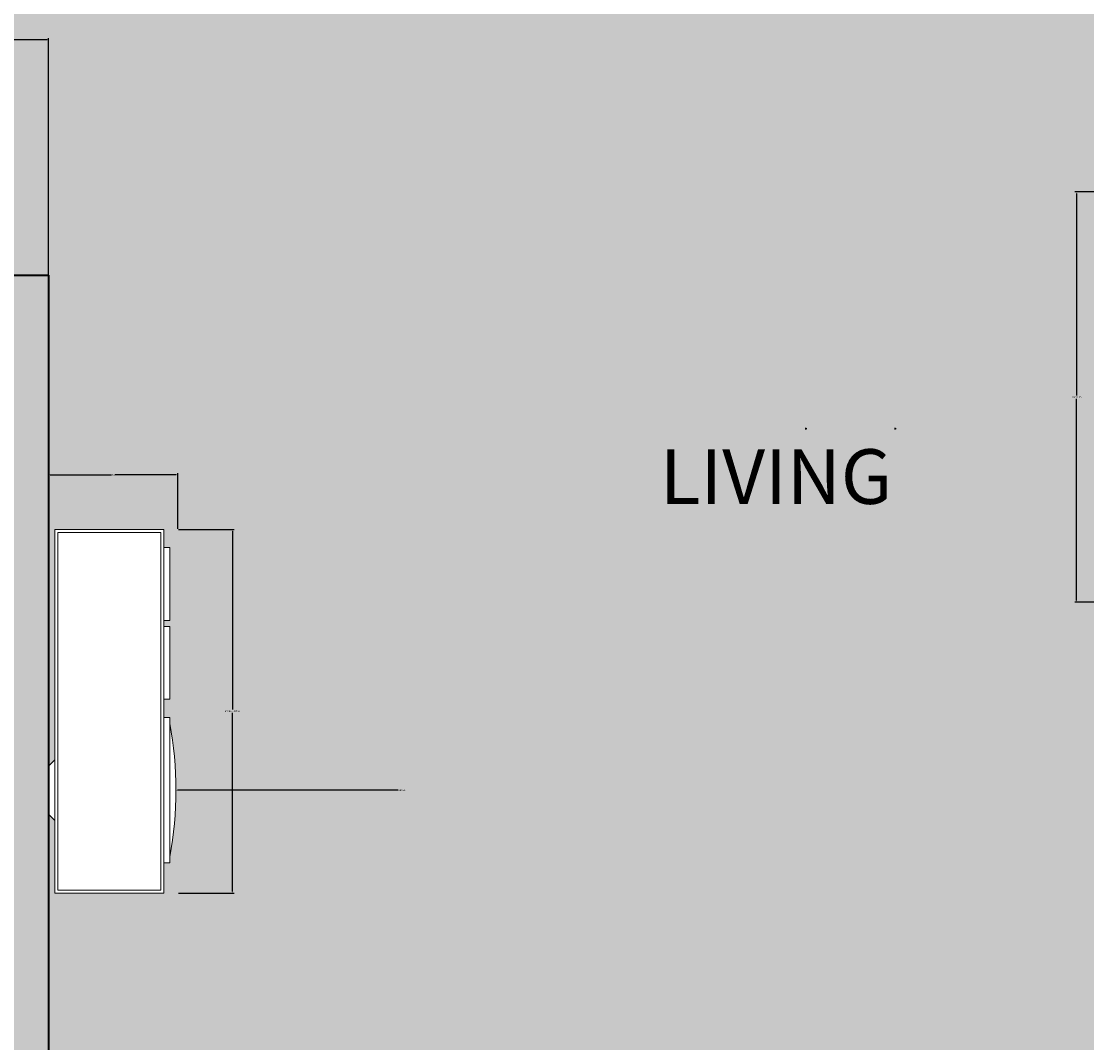
# Model space of a CAD drawing. Units: inches. Extents: x 3024 to 3952, y 1308 to 1863.
# Tile 5 of 29: x 3275 to 3392, y 1449 to 1560. Entities that reach past the tile are written whole.
import ezdxf

# ---------------------------------------------------------------- set-up
doc = ezdxf.new("R2010")
doc.units = ezdxf.units.IN
for name, color, linetype, lineweight in [('A-ANNO-DIMS', 2, 'Continuous', 18), ('A-AREA-IDEN', 7, 'Continuous', 18), ('A-FLOR-TILE-PATT', 7, 'Continuous', 13), ('A-FURN', 8, 'Continuous', 18), ('A-WALL', 7, 'Continuous', 35)]:
    doc.layers.add(name, color=color, linetype=linetype, lineweight=lineweight)
doc.layers.add('A-FLOR-PATT', color=254, linetype='Continuous', lineweight=13, true_color=0xfeeab9)
doc.layers.add('A-WALL-PATT', color=254, linetype='Continuous', lineweight=13, true_color=0xcecce6)
doc.styles.get("Standard").update_dxf_attribs({"font": 'arial.ttf'})
doc.dimstyles.get("Standard").update_dxf_attribs({"dimtxt": 0.18, "dimasz": 0.18, "dimexe": 0.18, "dimexo": 0.0625, "dimgap": 0.09, "dimtad": 0, "dimtih": 1, "dimtoh": 1, "dimdec": 4, "dimzin": 0, "dimdsep": 46, "dimtxsty": 'Standard', "dimcen": 0.09, "dimadec": 0, "dimazin": 0, "dimtfac": 1, "dimtdec": 4, "dimtofl": 0, "dimtmove": 0, "dimatfit": 3, "dimfxl": 1, "dimtolj": 1, "dimtzin": 0, "dimarcsym": 0})

# ---------------------------------------------------------------- blocks, each defined once
blk = doc.blocks.new('Entertainment Center')
for p, q in [((-4, 0), (-5, -1)), ((4, 0), (-4, 0)), ((5, -1), (4, 0)), ((-17, -19), (-17, -1)), ((-17, -1), (43, -1)), ((-16.5, -18.5), (-16.5, -1.5)), ((-16.5, -1.5), (42.5, -1.5)), ((42.5, -1.5), (42.5, -18.5)), ((43, -1), (43, -19)), ((43, -19), (-17, -19)), ((42.5, -18.5), (-16.5, -18.5)), ((-12, -20), (-12, -19)), ((12, -19), (12, -20)), ((15, -20), (15, -19)), ((27, -19), (27, -20)), ((28, -20), (28, -19)), ((40, -19), (40, -20)), ((12, -20), (-12, -20)), ((27, -20), (15, -20)), ((40, -20), (28, -20))]:
    blk.add_line(p, q)
blk.add_arc((0, 40), 61, 259.6111, 280.3889)
blk = doc.blocks.new('*D32')
at = {"layer": 'A-ANNO-DIMS', "color": 0, "lineweight": -2, "transparency": 16777216}
for p, q in [((3397.09, 1541.71), (3390.23, 1541.71)), ((3390.41, 1541.53), (3390.41, 1519.43)), ((3390.41, 1496.96), (3390.41, 1519.06)), ((3397.09, 1496.78), (3390.23, 1496.78))]:
    blk.add_line(p, q, dxfattribs=at)
at = {"layer": 'A-ANNO-DIMS', "color": 0, "transparency": 16777216}
for points in [[(3390.38, 1541.53), (3390.44, 1541.53), (3390.41, 1541.71)], [(3390.38, 1496.96), (3390.44, 1496.96), (3390.41, 1496.78)]]:
    blk.add_solid(points, dxfattribs=at)
at = {"layer": 'Defpoints', "color": 0, "transparency": 16777216}
for p in [(3397.15, 1541.71), (3390.41, 1496.78), (3397.15, 1496.78)]:
    blk.add_point(p, dxfattribs=at)
at = {"layer": 'A-ANNO-DIMS', "color": 0, "transparency": 16777216, "insert": (3390.41, 1519.25), "char_height": 0.18, "attachment_point": 5}
blk.add_mtext('\\A1;TABLE 45', dxfattribs=at)
blk = doc.blocks.new('*D34')
at = {"layer": 'A-ANNO-DIMS', "color": 0, "lineweight": -2, "transparency": 16777216}
for p, q in [((3292, 1504.74), (3298.09, 1504.74)), ((3297.91, 1504.56), (3297.91, 1485)), ((3297.91, 1465.07), (3297.91, 1484.64)), ((3292, 1464.89), (3298.09, 1464.89))]:
    blk.add_line(p, q, dxfattribs=at)
at = {"layer": 'A-ANNO-DIMS', "color": 0, "transparency": 16777216}
for points in [[(3297.88, 1504.56), (3297.94, 1504.56), (3297.91, 1504.74)], [(3297.88, 1465.07), (3297.94, 1465.07), (3297.91, 1464.89)]]:
    blk.add_solid(points, dxfattribs=at)
at = {"layer": 'Defpoints', "color": 0, "transparency": 16777216}
for p in [(3291.93, 1504.74), (3297.91, 1504.74), (3291.93, 1464.89)]:
    blk.add_point(p, dxfattribs=at)
at = {"layer": 'A-ANNO-DIMS', "color": 0, "transparency": 16777216, "insert": (3297.91, 1484.82), "char_height": 0.18, "attachment_point": 5}
blk.add_mtext('\\A1;MEDIA UNIT 40', dxfattribs=at)
blk = doc.blocks.new('*D35')
at = {"layer": 'A-ANNO-DIMS', "color": 0, "lineweight": -2, "transparency": 16777216}
for p, q in [((3277.76, 1504.8), (3277.76, 1510.9)), ((3291.93, 1504.8), (3291.93, 1510.9)), ((3277.94, 1510.72), (3284.64, 1510.72)), ((3291.75, 1510.72), (3285.06, 1510.72))]:
    blk.add_line(p, q, dxfattribs=at)
at = {"layer": 'A-ANNO-DIMS', "color": 0, "transparency": 16777216}
for points in [[(3277.94, 1510.75), (3277.94, 1510.69), (3277.76, 1510.72)], [(3291.75, 1510.75), (3291.75, 1510.69), (3291.93, 1510.72)]]:
    blk.add_solid(points, dxfattribs=at)
at = {"layer": 'Defpoints', "color": 0, "transparency": 16777216}
for p in [(3277.76, 1510.72), (3277.76, 1504.74), (3291.93, 1504.74)]:
    blk.add_point(p, dxfattribs=at)
at = {"layer": 'A-ANNO-DIMS', "color": 0, "transparency": 16777216, "insert": (3284.85, 1510.72), "char_height": 0.18, "attachment_point": 5}
blk.add_mtext('\\A1;14', dxfattribs=at)
blk = doc.blocks.new('*D65')
at = {"layer": 'A-ANNO-DIMS', "color": 0, "lineweight": -2, "transparency": 16777216}
for p, q in [((3262.76, 1532.67), (3262.76, 1558.56)), ((3262.94, 1558.38), (3269.81, 1558.38)), ((3277.58, 1558.38), (3270.72, 1558.38)), ((3277.76, 1532.67), (3277.76, 1558.56))]:
    blk.add_line(p, q, dxfattribs=at)
at = {"layer": 'A-ANNO-DIMS', "color": 0, "transparency": 16777216}
for points in [[(3262.94, 1558.41), (3262.94, 1558.35), (3262.76, 1558.38)], [(3277.58, 1558.41), (3277.58, 1558.35), (3277.76, 1558.38)]]:
    blk.add_solid(points, dxfattribs=at)
at = {"layer": 'Defpoints', "color": 0, "transparency": 16777216}
for p in [(3277.76, 1558.38), (3262.76, 1532.61), (3277.76, 1532.61)]:
    blk.add_point(p, dxfattribs=at)
at = {"layer": 'A-ANNO-DIMS', "color": 0, "transparency": 16777216, "insert": (3270.26, 1558.38), "char_height": 0.18, "attachment_point": 5}
blk.add_mtext('\\A1;15.003', dxfattribs=at)
blk = doc.blocks.new('*D104')
at = {"layer": 'A-ANNO-DIMS', "color": 0, "lineweight": -2, "transparency": 16777216}
for p, q in [((3360.65, 1515.79), (3360.83, 1515.79)), ((3360.74, 1515.7), (3360.74, 1515.88)), ((3507.36, 1515.79), (3452.55, 1515.79))]:
    blk.add_line(p, q, dxfattribs=at)
at = {"layer": 'A-ANNO-DIMS', "color": 0, "transparency": 16777216}
blk.add_solid([(3452.55, 1515.82), (3452.55, 1515.76), (3452.37, 1515.79)], dxfattribs=at)
at = {"layer": 'Defpoints', "color": 0, "transparency": 16777216}
for p in [(3360.74, 1515.79), (3452.37, 1515.79)]:
    blk.add_point(p, dxfattribs=at)
at = {"layer": 'A-ANNO-DIMS', "color": 0, "transparency": 16777216, "insert": (3507.83, 1515.79), "char_height": 0.18, "attachment_point": 5}
blk.add_mtext('\\A1;R91.64', dxfattribs=at)
blk = doc.blocks.new('*D105')
at = {"layer": 'A-ANNO-DIMS', "color": 0, "lineweight": -2, "transparency": 16777216}
for p, q in [((3370.44, 1515.79), (3370.62, 1515.79)), ((3370.53, 1515.7), (3370.53, 1515.88)), ((3508.74, 1515.79), (3457.09, 1515.79))]:
    blk.add_line(p, q, dxfattribs=at)
at = {"layer": 'A-ANNO-DIMS', "color": 0, "transparency": 16777216}
blk.add_solid([(3457.09, 1515.82), (3457.09, 1515.76), (3456.91, 1515.79)], dxfattribs=at)
at = {"layer": 'Defpoints', "color": 0, "transparency": 16777216}
for p in [(3370.53, 1515.79), (3456.91, 1515.79)]:
    blk.add_point(p, dxfattribs=at)
at = {"layer": 'A-ANNO-DIMS', "color": 0, "transparency": 16777216, "insert": (3509.22, 1515.79), "char_height": 0.18, "attachment_point": 5}
blk.add_mtext('\\A1;R86.38', dxfattribs=at)
blk = doc.blocks.new('*D106')
at = {"layer": 'A-ANNO-DIMS', "color": 0, "lineweight": -2, "transparency": 16777216}
for p, q in [((3251.11, 1476.18), (3251.29, 1476.18)), ((3251.2, 1476.09), (3251.2, 1476.27)), ((3316.02, 1476.18), (3291.89, 1476.18))]:
    blk.add_line(p, q, dxfattribs=at)
at = {"layer": 'A-ANNO-DIMS', "color": 0, "transparency": 16777216}
blk.add_solid([(3291.89, 1476.21), (3291.89, 1476.15), (3291.71, 1476.18)], dxfattribs=at)
at = {"layer": 'Defpoints', "color": 0, "transparency": 16777216}
for p in [(3251.2, 1476.18), (3291.71, 1476.18)]:
    blk.add_point(p, dxfattribs=at)
at = {"layer": 'A-ANNO-DIMS', "color": 0, "transparency": 16777216, "insert": (3316.48, 1476.18), "char_height": 0.18, "attachment_point": 5}
blk.add_mtext('\\A1;R40.51', dxfattribs=at)

msp = doc.modelspace()

# ---------------------------------------------------------------- hatches: boundary and pattern name
at = {"layer": 'A-FLOR-PATT', "transparency": 33554528}
h = msp.add_hatch(color=256, dxfattribs=at)
h.dxf.hatch_style = 1
h.paths.add_polyline_path([(3460.764, 1688.6064), (3412.764, 1688.6064), (3412.764, 1694.6064), (3460.764, 1694.6064), (3460.764, 1778.6064), (3406.764, 1778.6064), (3406.764, 1759.9514), (3318.2981, 1759.9514), (3318.2981, 1658.6064), (3322.5356, 1658.6064), (3322.5356, 1652.6064), (3292.764, 1652.6064), (3292.764, 1778.6064), (3106.764, 1778.6064), (3106.764, 1628.6064), (3172.764, 1628.6064), (3172.764, 1532.6064), (3166.764, 1532.6064), (3166.764, 1628.6064), (3106.764, 1628.6064), (3106.764, 1356.8452), (3202.812, 1356.8452), (3202.812, 1354.2534), (3202.812, 1353.8388), (3202.812, 1351.1212), (3202.812, 1347.8452), (3277.764, 1347.8452), (3277.764, 1353.8452), (3277.764, 1356.8452), (3277.764, 1442.6064), (3460.764, 1442.6064)])
h.paths.add_polyline_path([(3216.238, 1527.2064), (3216.238, 1491.2064), (3214.663, 1491.2064), (3214.663, 1491.2409, -0.39662236), (3180.243, 1526.6064), (3163.0285, 1526.6064), (3163.0285, 1531.1064), (3161.716, 1531.1064), (3161.716, 1561.1064), (3163.0285, 1561.1064), (3163.0285, 1531.1064), (3163.0285, 1526.6064), (3180.243, 1526.6064, 0.39662236), (3214.663, 1491.2409), (3214.663, 1527.2064)], flags=16)
h.paths.add_polyline_path([(3227.364, 1649.8972), (3191.364, 1649.8972), (3191.364, 1651.4722), (3227.364, 1651.4722)], flags=16)
h.paths.add_polyline_path([(3323.1172, 1606.7362), (3323.8545, 1606.8514), (3323.8545, 1594.8241), (3323.1172, 1594.9393)], flags=16)
h.paths.add_polyline_path([(3324.2232, 1606.909), (3330.1216, 1607.8307), (3330.1216, 1614.1093), (3339.3495, 1614.1093), (3340.2711, 1620.0078), (3352.4136, 1620.0078), (3353.3353, 1614.1093), (3359.9941, 1614.1093), (3360.9157, 1620.0078), (3373.0582, 1620.0078), (3373.9799, 1614.1093), (3383.2077, 1614.1093), (3383.2077, 1607.8307), (3389.1062, 1606.909), (3389.1062, 1594.7665), (3383.2077, 1593.8449), (3383.2077, 1587.5663), (3373.9799, 1587.5663), (3373.0583, 1581.6678), (3360.9157, 1581.6678), (3359.9941, 1587.5663), (3353.3353, 1587.5663), (3352.4136, 1581.6678), (3340.2711, 1581.6678), (3339.3495, 1587.5663), (3330.1216, 1587.5663), (3330.1216, 1593.8449), (3324.2232, 1594.7665)], flags=16)
h.paths.add_polyline_path([(3236.1584, 1693.1064), (3236.1584, 1723.1064), (3237.4709, 1723.1064), (3237.4709, 1693.1064)], flags=16)
h.paths.add_polyline_path([(3373.2158, 1600.6847), (3373.7965, 1600.7303), (3374.3268, 1600.7874), (3374.8132, 1600.8531), (3375.2621, 1600.9247), (3375.6801, 1600.9991), (3376.0736, 1601.0735), (3376.6855, 1601.19), (3377.366, 1601.3023), (3378.0667, 1601.3814), (3378.8026, 1601.4123), (3379.5865, 1601.3839), (3380.4537, 1601.2948), (3381.301, 1601.1717), (3382.0317, 1601.0433), (3382.4398, 1600.9607), (3382.6252, 1600.9201), (3382.919, 1600.8507), (3382.9044, 1600.8531), (3382.842, 1600.8678), (3382.7541, 1600.8896), (3382.6252, 1600.9201), (3382.4398, 1600.9607), (3382.1868, 1601.0119), (3381.8738, 1601.0711), (3381.5125, 1601.1346), (3381.1149, 1601.1988), (3380.6928, 1601.2601), (3380.2581, 1601.3149), (3379.8226, 1601.3597), (3379.3984, 1601.3908), (3378.9944, 1601.4054), (3378.6092, 1601.4042), (3378.2384, 1601.3886), (3377.8777, 1601.36), (3377.5227, 1601.32), (3377.1691, 1601.2698), (3376.8127, 1601.211), (3376.4491, 1601.145), (3376.0736, 1601.0735), (3375.4177, 1600.9494), (3374.5542, 1600.8119), (3373.5044, 1600.6988)], flags=0)
h.paths.add_polyline_path([(3380.0253, 1596.7351), (3380.499, 1596.6659), (3380.9706, 1596.6119), (3381.4375, 1596.5791), (3381.8971, 1596.5736), (3382.5886, 1596.6167), (3382.7848, 1596.6692), (3382.1465, 1596.5706), (3381.236, 1596.5815), (3380.3199, 1596.6865)], flags=0)
h.paths.add_polyline_path([(3369.6414, 1603.9617), (3370.1589, 1604.0021), (3370.6218, 1604.0539), (3371.0335, 1604.1173), (3371.3978, 1604.1921), (3371.7181, 1604.2785), (3371.9984, 1604.3761), (3372.2441, 1604.483), (3372.4611, 1604.5972), (3372.655, 1604.7163), (3372.8317, 1604.8384), (3372.9968, 1604.9611), (3373.3703, 1605.2455), (3373.8426, 1605.5328), (3374.4624, 1605.7539), (3375.1058, 1605.8302), (3375.7221, 1605.8261), (3376.4109, 1605.76), (3377.1534, 1605.6376), (3377.8945, 1605.473), (3378.1382, 1605.409), (3377.7394, 1605.5074), (3377.3509, 1605.5937), (3376.9704, 1605.6677), (3376.5999, 1605.7288), (3376.2417, 1605.7762), (3375.8979, 1605.8092), (3375.5707, 1605.8271), (3375.2621, 1605.8291), (3374.9745, 1605.8146), (3374.7092, 1605.7832), (3374.4647, 1605.7359), (3374.239, 1605.6742), (3374.0298, 1605.5996), (3373.835, 1605.5134), (3373.6525, 1605.4171), (3373.4801, 1605.3123), (3373.3156, 1605.2002), (3373.1562, 1605.0825), (3372.7603, 1604.781), (3372.236, 1604.4588), (3371.5738, 1604.2283), (3370.8493, 1604.0794), (3369.9262, 1603.976)], flags=0)
h.paths.add_polyline_path([(3366.7533, 1606.5832), (3367.1713, 1606.5519), (3367.5378, 1606.5374), (3367.8568, 1606.5394), (3368.1325, 1606.5573), (3368.3694, 1606.5903), (3368.5717, 1606.6377), (3368.7438, 1606.6988), (3368.89, 1606.7728), (3369.0146, 1606.8591), (3369.121, 1606.9568), (3369.2094, 1607.0646), (3369.2792, 1607.181), (3369.3295, 1607.3046), (3369.3596, 1607.4339), (3369.3688, 1607.5676), (3369.3565, 1607.7042), (3369.3218, 1607.8422), (3369.2649, 1607.9804), (3369.1893, 1608.1187), (3369.0993, 1608.2569), (3368.9992, 1608.3952), (3368.8934, 1608.5334), (3368.7861, 1608.6717), (3368.6817, 1608.8099), (3368.4212, 1609.1804), (3368.2685, 1609.7106), (3368.4883, 1610.1814), (3369.0537, 1610.4604), (3369.6717, 1610.5097), (3370.2812, 1610.3612), (3370.4805, 1610.2968), (3370.1882, 1610.3839), (3369.9284, 1610.4472), (3369.6905, 1610.4842), (3369.4662, 1610.4933), (3369.2555, 1610.4765), (3369.0608, 1610.4367), (3368.884, 1610.3767), (3368.7274, 1610.2994), (3368.5931, 1610.2077), (3368.4833, 1610.1045), (3368.4002, 1609.9927), (3368.3451, 1609.8747), (3368.3166, 1609.7517), (3368.3127, 1609.6244), (3368.331, 1609.4935), (3368.3696, 1609.3597), (3368.4261, 1609.2237), (3368.4985, 1609.0863), (3368.5845, 1608.9482), (3368.6817, 1608.8099), (3368.7861, 1608.6717), (3368.8934, 1608.5334), (3368.9992, 1608.3952), (3369.0993, 1608.2569), (3369.3398, 1607.8876), (3369.3941, 1607.2896), (3368.9774, 1606.7817), (3368.3928, 1606.5742), (3367.7162, 1606.5303), (3367.0044, 1606.5585)], flags=0)
h.paths.add_polyline_path([(3362.1859, 1610.2589), (3362.5478, 1610.2845), (3362.8348, 1610.3275), (3363.0585, 1610.3863), (3363.2303, 1610.4595), (3363.3619, 1610.5457), (3363.463, 1610.6432), (3363.5376, 1610.7502), (3363.5876, 1610.8643), (3363.6153, 1610.9834), (3363.6229, 1611.1055), (3363.6125, 1611.2283), (3363.5861, 1611.3496), (3363.5462, 1611.4673), (3363.4949, 1611.5797), (3363.4358, 1611.6871), (3363.3723, 1611.7902), (3363.3081, 1611.8897), (3363.2468, 1611.9863), (3363.192, 1612.0808), (3363.0258, 1612.4261), (3363.3371, 1612.8672), (3363.9008, 1612.9782), (3364.4822, 1612.9641), (3365.1098, 1612.9074), (3365.328, 1612.8805), (3364.9615, 1612.9208), (3364.6426, 1612.9496), (3364.3668, 1612.9669), (3364.1299, 1612.9726), (3363.9276, 1612.9669), (3363.7555, 1612.9496), (3363.6093, 1612.9208), (3363.4848, 1612.8805), (3363.3782, 1612.8289), (3363.2889, 1612.7672), (3363.2169, 1612.6969), (3363.1622, 1612.6193), (3363.1247, 1612.5361), (3363.1046, 1612.4484), (3363.1017, 1612.358), (3363.1161, 1612.266), (3363.1472, 1612.1738), (3363.192, 1612.0808), (3363.2468, 1611.9863), (3363.3081, 1611.8897), (3363.3723, 1611.7902), (3363.4358, 1611.6871), (3363.6363, 1611.323), (3363.5979, 1610.7003), (3363.0863, 1610.3651), (3362.3983, 1610.2622)], flags=0)
h.paths.add_polyline_path([(3352.356, 1581.2991), (3352.2408, 1580.5618), (3340.4439, 1580.5618), (3340.3287, 1581.2991)], flags=16)
h.paths.add_polyline_path([(3340.4439, 1621.1137), (3352.2408, 1621.1137), (3352.356, 1620.3764), (3340.3287, 1620.3764)], flags=16)
h.paths.add_polyline_path([(3278.4282, 1504.7424), (3290.3831, 1504.7424), (3290.3831, 1502.7499), (3291.0473, 1502.7499), (3291.0473, 1494.7799), (3290.3831, 1494.7799), (3290.3831, 1494.1158), (3291.0473, 1494.1158), (3291.0473, 1486.1458), (3290.3831, 1486.1458), (3290.3831, 1484.1533), (3291.0473, 1484.1533), (3291.0473, 1483.4892, -0.09090909), (3291.0473, 1468.8776), (3291.0473, 1468.2135), (3290.3831, 1468.2135), (3290.3831, 1464.8926), (3278.4282, 1464.8926), (3278.4282, 1472.8626), (3277.764, 1473.5268), (3277.764, 1478.84), (3278.4282, 1479.5042)], flags=16)
h.paths.add_polyline_path([(3278.7603, 1504.4103), (3290.051, 1504.4103), (3290.051, 1465.2247), (3278.7603, 1465.2247)], flags=0)
h.paths.add_polyline_path([(3123.904, 1600.7821), (3117.9039, 1602.7821), (3117.9039, 1599.7821), (3119.4039, 1599.7821), (3119.4039, 1596.7821), (3118.4039, 1596.7821), (3118.4039, 1598.7821), (3117.9039, 1598.7821), (3117.9039, 1596.2821), (3109.9039, 1596.2821), (3109.9039, 1617.2821), (3117.9039, 1617.2821), (3117.9039, 1610.7821), (3123.9038, 1612.7821, -0.70257121), (3137.9039, 1606.7822, -0.70256205)], flags=16)
h.paths.add_polyline_path([(3123.9039, 1602.7822), (3123.9039, 1610.7822, -0.73453329), (3136.9039, 1606.7822, -0.73452973)], flags=0)
h.paths.add_polyline_path([(3177.972, 1689.6473), (3109.2405, 1689.6473), (3109.2405, 1741.1959), (3177.972, 1741.1959)], flags=16)
h.paths.add_polyline_path([(3373.0006, 1581.2991), (3372.8854, 1580.5618), (3361.0885, 1580.5618), (3360.9733, 1581.2991)], flags=16)
h.paths.add_polyline_path([(3361.0885, 1621.1137), (3372.8854, 1621.1137), (3373.0006, 1620.3764), (3360.9733, 1620.3764)], flags=16)
h.paths.add_polyline_path([(3116.9039, 1598.2821, -0.41421356), (3116.1539, 1597.2821), (3111.9039, 1597.2821, -0.41421356), (3110.9039, 1598.0321), (3110.9039, 1615.2821, -0.41421356), (3111.6539, 1616.2821), (3115.9039, 1616.2821, -0.41421356), (3116.9039, 1615.5321)], flags=0)
h.paths.add_polyline_path([(3121.6122, 1728.1369), (3121.6122, 1696.5205), (3110.2715, 1696.5205), (3110.2715, 1714.3906), (3121.6122, 1714.3906), (3121.6122, 1716.4526), (3110.2715, 1716.4526), (3110.2715, 1734.3228), (3123.3304, 1734.3228), (3123.3304, 1729.8552), (3134.6711, 1741.1959), (3134.6711, 1728.1369)], flags=0)
h.paths.add_polyline_path([(3389.4748, 1606.8514), (3390.2122, 1606.7362), (3390.2122, 1594.9393), (3389.4748, 1594.8241)], flags=16)
h.paths.add_polyline_path([(3257.6842, 1762.8281), (3259.6842, 1768.8281), (3256.6842, 1768.8281), (3256.6842, 1767.3281), (3253.6842, 1767.3281), (3253.6842, 1768.3281), (3255.6842, 1768.3281), (3255.6842, 1768.8281), (3253.1842, 1768.8281), (3253.1842, 1776.8281), (3274.1842, 1776.8281), (3274.1842, 1768.8281), (3267.6842, 1768.8281), (3269.6842, 1762.8282, -0.70257121), (3263.6843, 1748.8282, -0.70256205)], flags=16)
h.paths.add_polyline_path([(3259.6842, 1762.8281), (3267.6843, 1762.8281, -0.73453329), (3263.6842, 1749.8282, -0.73452973)], flags=0)
h.paths.add_polyline_path([(3411.264, 1715.6064), (3411.264, 1716.9189), (3441.264, 1716.9189), (3441.264, 1715.6064)], flags=16)
h.paths.add_polyline_path([(3178.3806, 1449.1876), (3178.3806, 1397.639), (3109.6491, 1397.639), (3109.6491, 1449.1876)], flags=16)
h.paths.add_polyline_path([(3397.1501, 1541.7146), (3419.6183, 1541.7146), (3419.6183, 1496.7783), (3397.1501, 1496.7783)], flags=16)
h.paths.add_polyline_path([(3254.1842, 1770.5781), (3254.1842, 1774.8281, -0.41421356), (3254.9342, 1775.8281), (3272.1842, 1775.8281, -0.41421356), (3273.1842, 1775.0781), (3273.1842, 1770.8281, -0.41421356), (3272.4342, 1769.8281), (3255.1842, 1769.8281, -0.41421356)], flags=0)
h.paths.add_polyline_path([(3403.672, 1500.7601), (3403.6016, 1500.3997), (3403.5328, 1500.0441), (3403.4662, 1499.6867), (3403.4027, 1499.3226), (3403.3464, 1498.9532), (3403.3025, 1498.5811), (3403.2759, 1498.2091), (3403.2714, 1497.8401), (3403.3064, 1497.2813), (3403.3491, 1497.1219), (3403.2689, 1497.6395), (3403.2778, 1498.3719), (3403.3635, 1499.0984), (3403.4889, 1499.8168), (3403.6016, 1500.3997), (3403.672, 1500.7601), (3403.744, 1501.1315), (3403.817, 1501.5205), (3403.891, 1501.9336), (3403.9656, 1502.3769), (3404.0404, 1502.8572), (3404.115, 1503.3786), (3404.2264, 1504.2311), (3404.2571, 1504.5223), (3404.1552, 1503.6598), (3404.0063, 1502.6193), (3403.8604, 1501.7518), (3403.744, 1501.1315)], flags=0)
h.paths.add_polyline_path([(3406.5868, 1505.0416), (3406.6121, 1504.5236), (3406.6492, 1504.0526), (3406.6956, 1503.624), (3406.7491, 1503.2333), (3406.8072, 1502.8759), (3406.8676, 1502.5473), (3406.9281, 1502.243), (3407.0268, 1501.7597), (3407.1416, 1501.1368), (3407.2087, 1500.3904), (3407.1804, 1499.6703), (3407.1078, 1498.9956), (3407.0074, 1498.3199), (3406.8809, 1497.6059), (3406.7403, 1496.9627), (3406.7418, 1496.9824), (3406.7491, 1497.0249), (3406.8229, 1497.3409), (3406.8364, 1497.4025), (3406.878, 1497.6078), (3406.9261, 1497.8614), (3406.9777, 1498.1526), (3407.0298, 1498.4712), (3407.0797, 1498.8068), (3407.1243, 1499.149), (3407.1607, 1499.4874), (3407.1859, 1499.8115), (3407.1978, 1500.1137), (3407.1969, 1500.3962), (3407.1841, 1500.6642), (3407.1609, 1500.9225), (3407.1284, 1501.1761), (3407.0876, 1501.43), (3407.0398, 1501.6891), (3406.9862, 1501.9585), (3406.8832, 1502.4628), (3406.7712, 1503.0713), (3406.6657, 1503.8424), (3406.5924, 1504.7735)], flags=0)
h.paths.add_polyline_path([(3409.2517, 1507.8962), (3409.2752, 1507.4282), (3409.3079, 1507.0076), (3409.3501, 1506.6314), (3409.4015, 1506.2969), (3409.4624, 1506.0009), (3409.5326, 1505.7406), (3409.6119, 1505.5128), (3409.6988, 1505.3131), (3409.7915, 1505.1368), (3409.8883, 1504.9792), (3409.9875, 1504.8356), (3410.0872, 1504.7015), (3410.1859, 1504.572), (3410.4508, 1504.2132), (3410.7205, 1503.6035), (3410.8059, 1502.8824), (3410.7619, 1502.0875), (3410.6122, 1501.2299), (3410.4402, 1500.6169), (3410.2538, 1500.0031), (3410.0536, 1499.3219), (3409.9909, 1499.0812), (3410.1761, 1499.7472), (3410.3596, 1500.3513), (3410.4512, 1500.6561), (3410.5312, 1500.9412), (3410.6013, 1501.226), (3410.6614, 1501.512), (3410.7111, 1501.7964), (3410.7496, 1502.0763), (3410.7764, 1502.3489), (3410.7909, 1502.6114), (3410.7926, 1502.8608), (3410.7808, 1503.0944), (3410.7553, 1503.31), (3410.7169, 1503.5087), (3410.6667, 1503.6921), (3410.6061, 1503.8621), (3410.5361, 1504.0203), (3410.4578, 1504.1686), (3410.3726, 1504.3088), (3410.2815, 1504.4424), (3410.1859, 1504.572), (3410.0872, 1504.7015), (3409.859, 1505.0083), (3409.5943, 1505.5117), (3409.4266, 1506.1336), (3409.324, 1506.8011), (3409.2586, 1507.6407)], flags=0)
h.paths.add_polyline_path([(3411.4914, 1510.5878), (3411.4432, 1510.1586), (3411.4054, 1509.775), (3411.38, 1509.4354), (3411.3681, 1509.1376), (3411.3698, 1508.8784), (3411.3843, 1508.6542), (3411.4112, 1508.4618), (3411.4497, 1508.2974), (3411.4994, 1508.1575), (3411.5595, 1508.0388), (3411.6296, 1507.9375), (3411.7097, 1507.851), (3411.802, 1507.7792), (3411.9096, 1507.7225), (3412.0353, 1507.6817), (3412.1821, 1507.6572), (3412.3528, 1507.6496), (3412.5505, 1507.6597), (3412.778, 1507.6879), (3413.0364, 1507.7341), (3413.3194, 1507.7955), (3413.6188, 1507.8687), (3413.9264, 1507.95), (3414.234, 1508.036), (3414.5333, 1508.1232), (3414.8163, 1508.208), (3415.0747, 1508.287), (3415.3023, 1508.3569), (3415.5007, 1508.4158), (3415.6733, 1508.4617), (3416.1158, 1508.5538), (3416.512, 1508.2591), (3416.716, 1507.6581), (3416.61, 1507.0003), (3416.3052, 1506.3411), (3415.8928, 1505.618), (3415.7339, 1505.3633), (3415.9914, 1505.791), (3416.201, 1506.1583), (3416.3666, 1506.4739), (3416.4925, 1506.7462), (3416.5828, 1506.9838), (3416.6413, 1507.1949), (3416.6725, 1507.3883), (3416.6799, 1507.5705), (3416.6662, 1507.7417), (3416.6339, 1507.9), (3416.5851, 1508.0436), (3416.5223, 1508.1709), (3416.4478, 1508.28), (3416.3639, 1508.3692), (3416.273, 1508.4368), (3416.1765, 1508.4815), (3416.0718, 1508.5047), (3415.9553, 1508.5079), (3415.8237, 1508.493), (3415.6733, 1508.4617), (3415.5007, 1508.4158), (3415.3327, 1508.3659), (3414.6495, 1508.157), (3414.0606, 1507.9855), (3413.4456, 1507.8229), (3412.8838, 1507.701), (3412.5505, 1507.6597), (3412.0748, 1507.6354), (3411.595, 1507.8883), (3411.398, 1508.4429), (3411.3624, 1508.9927), (3411.3854, 1509.5711), (3411.4578, 1510.3071)], flags=0)
h.paths.add_polyline_path([(3135.0797, 1449.1876), (3135.0797, 1436.1286), (3122.0208, 1436.1286), (3122.0208, 1404.5122), (3110.6801, 1404.5122), (3110.6801, 1422.3823), (3122.0208, 1422.3823), (3122.0208, 1424.4443), (3110.6801, 1424.4443), (3110.6801, 1442.3145), (3123.739, 1442.3145), (3123.739, 1437.8469)], flags=0)
h.paths.add_polyline_path([(3416.4944, 1514.2949), (3416.4837, 1513.8511), (3416.4893, 1513.4867), (3416.5102, 1513.1926), (3416.5451, 1512.9593), (3416.5929, 1512.7775), (3416.6524, 1512.6379), (3416.7224, 1512.531), (3416.8017, 1512.4488), (3416.8886, 1512.3882), (3416.9813, 1512.3476), (3417.0781, 1512.3251), (3417.1773, 1512.3189), (3417.277, 1512.3274), (3417.3757, 1512.3488), (3417.4713, 1512.3813), (3417.5627, 1512.4229), (3417.65, 1512.471), (3417.7338, 1512.5225), (3417.8146, 1512.5747), (3417.8931, 1512.6245), (3417.9699, 1512.6691), (3418.2968, 1512.8265), (3418.6505, 1512.4645), (3418.7037, 1511.9342), (3418.6693, 1511.3839), (3418.6076, 1510.8228), (3418.5777, 1510.5927), (3418.6197, 1510.9333), (3418.6525, 1511.2311), (3418.6759, 1511.4903), (3418.6899, 1511.7144), (3418.6946, 1511.9069), (3418.6899, 1512.0713), (3418.6759, 1512.2112), (3418.6525, 1512.33), (3418.6197, 1512.4311), (3418.5778, 1512.5177), (3418.5276, 1512.5903), (3418.4705, 1512.6488), (3418.4075, 1512.6933), (3418.3399, 1512.7237), (3418.2686, 1512.7401), (3418.1951, 1512.7424), (3418.1204, 1512.7307), (3418.0455, 1512.7055), (3417.9792, 1512.6736), (3417.65, 1512.471), (3417.5627, 1512.4229), (3417.4713, 1512.3813), (3417.3757, 1512.3488), (3417.277, 1512.3274), (3416.878, 1512.2936), (3416.5757, 1512.7549), (3416.492, 1513.3145), (3416.4808, 1514.0384)], flags=0)
h.paths.add_polyline_path([(3392.8223, 1481.9454), (3396.7707, 1481.9454), (3396.7707, 1480.9201), (3428.3585, 1480.9201), (3428.3585, 1481.9454), (3432.3069, 1481.9454), (3432.3069, 1464.8354, -0.26666697), (3392.8223, 1464.8354)], flags=16)
h.paths.add_polyline_path([(3431.203, 1547.5428), (3450.8613, 1547.5428, -0.19047621), (3450.8614, 1484.031), (3431.203, 1484.031), (3431.203, 1488.5675), (3432.3809, 1488.5675), (3432.3809, 1543.0062), (3431.203, 1543.0062)], flags=16)
h.paths.add_polyline_path([(3451.9233, 1524.86, -0.04962821), (3451.9233, 1506.7138), (3446.7921, 1506.7138), (3446.7921, 1524.86)], flags=0)
h.paths.add_polyline_path([(3460.764, 1436.6064), (3277.764, 1436.6064), (3277.764, 1356.8452), (3277.764, 1353.8452), (3460.764, 1353.8452)], flags=17)
h.paths.add_polyline_path([(3121.3033, 1577.378), (3153.693, 1577.378), (3153.693, 1586.6752), (3121.3033, 1586.6752)], flags=24)
h.paths.add_polyline_path([(3164.1457, 1464.1276), (3210.4801, 1464.1276), (3210.4801, 1473.4247), (3164.1457, 1473.4247)], flags=24)
h.paths.add_polyline_path([(3343.1909, 1505.8863), (3373.7236, 1505.8863), (3373.7236, 1515.1773), (3343.1909, 1515.1773)], flags=24)
h.paths.add_polyline_path([(3337.6353, 1564.2926), (3370.0189, 1564.2926), (3370.0189, 1573.5836), (3337.6353, 1573.5836)], flags=24)
h.paths.add_polyline_path([(3419.204, 1753.8578), (3453.3997, 1753.8578), (3453.3997, 1762.9956), (3419.204, 1762.9956)], flags=24)
h.paths.add_polyline_path([(3341.2523, 1701.0246), (3381.0761, 1701.0246), (3381.0761, 1710.3156), (3341.2523, 1710.3156)], flags=24)
h.paths.add_polyline_path([(3245.8895, 1726.2997), (3278.2793, 1726.2997), (3278.2793, 1735.5968), (3245.8895, 1735.5968)], flags=24)
h.paths.add_polyline_path([(3128.8045, 1668.6736), (3175.1389, 1668.6736), (3175.1389, 1677.9707), (3128.8045, 1677.9707)], flags=24)
h.paths.add_polyline_path([(3345.9997, 1396.0062), (3389.09, 1396.0062), (3389.09, 1405.3033), (3345.9997, 1405.3033)], flags=24)
at = {"layer": 'A-FLOR-TILE-PATT', "transparency": 33554569}
h = msp.add_hatch(dxfattribs=at)
h.set_pattern_fill('ANGLE', color=256, scale=2)
h.set_pattern_definition([(0, (0, 0), (0, 13.97), [10.16, -3.81]), (90, (0, 0), (-13.97, 9e-16), [10.16, -3.81])])
h.paths.add_polyline_path([(3292.764, 1778.6064), (3232.764, 1778.6064), (3232.764, 1694.6064), (3236.1584, 1694.6064), (3236.1584, 1723.1064), (3237.4709, 1723.1064), (3237.4709, 1723.0777, -0.38700389), (3266.1209, 1694.6064), (3292.764, 1694.6064)])
h.paths.add_polyline_path([(3263.6843, 1748.8282, -0.70256205), (3257.6842, 1762.8281), (3259.6842, 1768.8281), (3256.6842, 1768.8281), (3256.6842, 1767.3281), (3253.6842, 1767.3281), (3253.6842, 1768.3281), (3255.6842, 1768.3281), (3255.6842, 1768.8281), (3253.1842, 1768.8281), (3253.1842, 1776.8281), (3274.1842, 1776.8281), (3274.1842, 1768.8281), (3267.6842, 1768.8281), (3269.6842, 1762.8282, -0.70257121)], flags=16)
h.paths.add_polyline_path([(3263.6842, 1749.8282, -0.73452973), (3259.6842, 1762.8281), (3267.6843, 1762.8281, -0.73453329)], flags=0)
h.paths.add_polyline_path([(3255.1842, 1769.8281, -0.41421356), (3254.1842, 1770.5781), (3254.1842, 1774.8281, -0.41421356), (3254.9342, 1775.8281), (3272.1842, 1775.8281, -0.41421356), (3273.1842, 1775.0781), (3273.1842, 1770.8281, -0.41421356), (3272.4342, 1769.8281)], flags=0)
h.paths.add_polyline_path([(3460.764, 1436.6064), (3277.764, 1436.6064), (3277.764, 1356.8452), (3277.764, 1353.8452), (3460.764, 1353.8452)])
h.paths.add_polyline_path([(3166.764, 1628.6064), (3106.764, 1628.6064), (3106.764, 1532.6064), (3133.066, 1532.6064, -0.38700389), (3161.716, 1561.0777), (3161.716, 1561.1064), (3163.0285, 1561.1064), (3163.0285, 1532.6064), (3166.764, 1532.6064)])
h.paths.add_polyline_path([(3123.904, 1600.7821), (3117.9039, 1602.7821), (3117.9039, 1599.7821), (3119.4039, 1599.7821), (3119.4039, 1596.7821), (3118.4039, 1596.7821), (3118.4039, 1598.7821), (3117.9039, 1598.7821), (3117.9039, 1596.2821), (3109.9039, 1596.2821), (3109.9039, 1617.2821), (3117.9039, 1617.2821), (3117.9039, 1610.7821), (3123.9038, 1612.7821, -0.70257121), (3137.9039, 1606.7822, -0.70256205)], flags=16)
h.paths.add_polyline_path([(3123.9039, 1602.7822), (3123.9039, 1610.7822, -0.73453329), (3136.9039, 1606.7822, -0.73452973)], flags=0)
h.paths.add_polyline_path([(3116.1539, 1597.2821), (3111.9039, 1597.2821, -0.41421356), (3110.9039, 1598.0321), (3110.9039, 1615.2821, -0.41421356), (3111.6539, 1616.2821), (3115.9039, 1616.2821, -0.41421356), (3116.9039, 1615.5321), (3116.9039, 1598.2821, -0.41421356)], flags=0)
h.paths.add_polyline_path([(3245.8895, 1726.2997), (3278.2793, 1726.2997), (3278.2793, 1735.5968), (3245.8895, 1735.5968)], flags=24)
h.paths.add_polyline_path([(3345.9997, 1396.0062), (3389.09, 1396.0062), (3389.09, 1405.3033), (3345.9997, 1405.3033)], flags=24)
h.paths.add_polyline_path([(3121.3033, 1577.378), (3153.693, 1577.378), (3153.693, 1586.6752), (3121.3033, 1586.6752)], flags=24)
at = {"layer": 'A-WALL-PATT'}
h = msp.add_hatch(color=256, dxfattribs=at)
h.dxf.hatch_style = 1
h.paths.add_polyline_path([(3106.764, 1778.6064), (3140.5977, 1778.6064), (3140.5977, 1781.8824), (3140.5977, 1784.6), (3140.5977, 1787.6064), (3097.764, 1787.6064), (3097.764, 1590.213), (3101.04, 1590.213), (3103.7576, 1590.213), (3106.764, 1590.213)])
h.paths.add_polyline_path([(3253.5314, 1781.8824), (3253.5314, 1784.6), (3253.5314, 1787.6064), (3194.6826, 1787.6064), (3194.6826, 1785.0146), (3194.6826, 1784.6), (3194.6826, 1781.8824), (3194.6826, 1778.6064), (3253.5314, 1778.6064)])
h.paths.add_polyline_path([(3333.856, 1782.2838), (3333.856, 1784.7474), (3333.856, 1787.6064), (3272.0523, 1787.6064), (3272.0523, 1785.0146), (3272.0523, 1784.6), (3272.0523, 1781.8824), (3272.0523, 1778.6064), (3333.856, 1778.6064)])
h.paths.add_polyline_path([(3428.8344, 1784.6), (3428.8344, 1787.6064), (3378.3947, 1787.6064), (3378.3947, 1784.7474), (3378.3947, 1782.2838), (3378.3947, 1778.6064), (3428.8344, 1778.6064), (3428.8344, 1781.8824)], flags=17)
h.paths.add_polyline_path([(3469.764, 1787.6064), (3451.9386, 1787.6064), (3451.9386, 1785.0146), (3451.9386, 1784.6), (3451.9386, 1781.8824), (3451.9386, 1778.6064), (3460.764, 1778.6064), (3460.764, 1353.8452), (3277.764, 1353.8452), (3277.764, 1347.8452), (3469.764, 1347.8452), (3469.764, 1353.8452)])
h.paths.add_polyline_path([(3106.764, 1571.6922), (3104.1722, 1571.6922), (3103.7576, 1571.6922), (3101.04, 1571.6922), (3097.764, 1571.6922), (3097.764, 1347.8452), (3148.7271, 1347.8452), (3148.7271, 1351.1212), (3148.7271, 1353.8388), (3148.7271, 1356.8452), (3106.764, 1356.8452)])
h.paths.add_polyline_path([(3277.764, 1532.6064), (3262.7605, 1532.6064), (3262.7605, 1582.9359), (3256.7605, 1582.9359), (3256.7605, 1532.6064), (3244.2116, 1532.6064), (3216.238, 1532.6064), (3216.238, 1527.2064), (3216.238, 1526.6064), (3271.764, 1526.6064), (3271.764, 1356.8452), (3202.812, 1356.8452), (3202.812, 1354.2534), (3202.812, 1353.8388), (3202.812, 1351.1212), (3202.812, 1347.8452), (3277.764, 1347.8452), (3277.764, 1353.8452), (3277.764, 1356.8452)])
h.paths.add_polyline_path([(3180.238, 1532.6064), (3163.0285, 1532.6064), (3163.0285, 1531.1064), (3163.0285, 1526.6064), (3180.243, 1526.6064, -0.00416688), (3180.238, 1527.2064)])
h.paths.add_polyline_path([(3133.0285, 1531.1064, -0.01250587), (3133.066, 1532.6064), (3106.764, 1532.6064), (3106.764, 1526.6064), (3133.0285, 1526.6064)], flags=17)
h.paths.add_polyline_path([(3172.764, 1628.6064), (3166.764, 1628.6064), (3166.764, 1532.6064), (3172.764, 1532.6064)])
h.paths.add_polyline_path([(3232.764, 1649.8972), (3227.364, 1649.8972), (3226.764, 1649.8972), (3226.764, 1634.6064), (3106.764, 1634.6064), (3106.764, 1628.6064), (3232.764, 1628.6064)])

# ---------------------------------------------------------------- linework, layer by layer
at = {"layer": 'A-WALL'}
for p in [(3262.7605, 1532.6064), (3277.764, 1356.8452)]:
    msp.add_line(p, (3277.764, 1532.6064), dxfattribs=at)

# ---------------------------------------------------------------- block references
at = {"layer": 'A-FURN', "xscale": 0.6641619615054923, "yscale": 0.6641619615054923, "zscale": 0.6641619615054923, "rotation": 90}
msp.add_blockref('Entertainment Center', (3277.764, 1476.1834), dxfattribs=at)

# ---------------------------------------------------------------- texts
at = {"layer": 'A-AREA-IDEN'}
msp.add_text('LIVING', height=5.98971, dxfattribs=at).set_placement((3344.7394, 1507.537))

# ---------------------------------------------------------------- dimensions: what is measured, and where the dimension line sits
at = {"layer": 'A-ANNO-DIMS'}
dim = msp.add_linear_dim(base=(3277.76402, 1558.38141), p1=(3262.76054, 1532.6064), p2=(3277.76402, 1532.6064), dimstyle='Standard', override={"dimdec": 3, "dimlfac": 1, "dimrnd": 0, "dimzin": 0, "dimdsep": 46, "dimlunit": 2}, dxfattribs=at)
dim.commit()
dim.dimension.update_dxf_attribs({"geometry": '*D65', "text_midpoint": (3270.26228, 1558.38141)})
for base, p1, p2, angle, text, picture, middle in [((3390.4097, 1496.7783), (3397.1501, 1541.7146), (3397.1501, 1496.7783), 270, 'TABLE <>', '*D32', (3390.4097, 1519.2465)), ((3297.9103, 1504.7424), (3291.9328, 1464.8926), (3291.9328, 1504.7424), 90, 'MEDIA UNIT <>', '*D34', (3297.9103, 1484.8175))]:
    dim = msp.add_linear_dim(base=base, p1=p1, p2=p2, angle=angle, text=text, dimstyle='Standard', override={"dimdec": 0, "dimlfac": 1, "dimrnd": 0, "dimzin": 0, "dimdsep": 46, "dimlunit": 2}, dxfattribs=at)
    dim.commit()
    dim.dimension.update_dxf_attribs({"geometry": picture, "text_midpoint": middle})
for center, mpoint, picture, middle in [((3360.7376, 1515.7869), (3452.3735, 1515.787), '*D104', (3507.3551, 1515.7871)), ((3370.5265, 1515.7869), (3456.9101, 1515.787), '*D105', (3508.7402, 1515.7871)), ((3251.1975, 1476.1834), (3291.7114, 1476.183), '*D106', (3316.0197, 1476.1828))]:
    dim = msp.add_radius_dim(center=center, mpoint=mpoint, dimstyle='Standard', override={"dimdec": 2, "dimlfac": 1, "dimrnd": 0, "dimzin": 0, "dimdsep": 46, "dimlunit": 2}, dxfattribs=at)
    dim.commit()
    dim.dimension.update_dxf_attribs({"geometry": picture, "text_midpoint": middle, "dimtype": 164})
dim = msp.add_linear_dim(base=(3277.764, 1510.7198), p1=(3291.9328, 1504.7424), p2=(3277.764, 1504.7424), angle=180, dimstyle='Standard', override={"dimdec": 0, "dimlfac": 1, "dimrnd": 0, "dimzin": 0, "dimdsep": 46, "dimlunit": 2}, dxfattribs=at)
dim.commit()
dim.dimension.update_dxf_attribs({"geometry": '*D35', "text_midpoint": (3284.8484, 1510.7198)})

doc.saveas('drawing.dxf')
